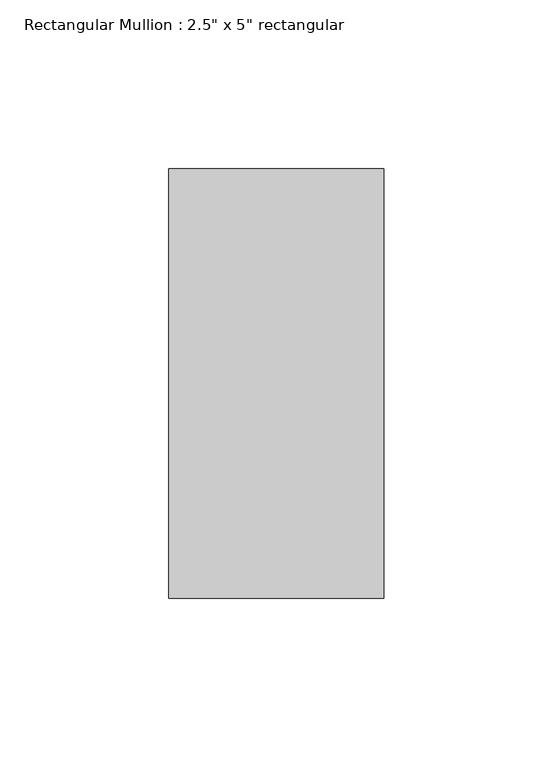
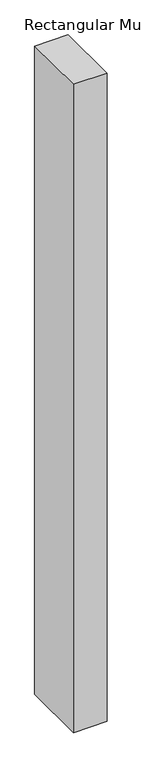
"""IFC4 building model written with IfcOpenShell, lengths in millimetres: member geometry."""

from ifc_helpers import new_model, si_unit, frame, origin, place, context, project, spatial, polyline, outline, extrude, source, transform, mapped, element, save


def member_9a0024e4(model_context):
    return source(origin(), model_context, "Body", "SweptSolid", [
        extrude(outline(polyline([(0.0, 63.5), (0.0, -63.5), (-63.5, -63.5), (-63.5, 63.5), (0.0, 63.5)])), frame((0.0, 0.0, -1299.6333333), z_axis=(0.0, 0.0, 1.0), x_axis=(1.0, 0.0, 0.0)), (0.0, 0.0, 1.0), 1299.6333333),
    ])


if __name__ == "__main__":
    model = new_model("IFC4")
    model_context = context("Model", 3, world=origin())
    ifc_project = project(units=[si_unit("LENGTHUNIT", "METRE", prefix="MILLI")], contexts=[model_context])
    site = spatial("IfcSite", under=ifc_project)
    building = spatial("IfcBuilding", under=site)
    placement = place(None, origin())
    member_shape = member_9a0024e4(model_context)
    element("IfcMember", 1, ObjectType="Rectangular Mullion : 2.5\" x 5\" rectangular", at=placement, inside=building, context=model_context, shape_type="MappedRepresentation", body=[
        mapped(member_shape, transform((0.0, 0.0, 0.0), x_axis=(1.0, 0.0, 0.0), y_axis=(0.0, 1.0, 0.0), z_axis=(0.0, 0.0, 1.0))),
    ])
    save(model, "model.ifc")

# Revit data of these elements
# Type "Rectangular Mullion : 2.5\" x 5\" rectangular"
#   built-in parameter 1007304 = 0.416667 (stored number, unit not read)
#   built-in parameter 1007301 = 0.104167 (stored number, unit not read)
#   built-in parameter 1007300 = 0.104167 (stored number, unit not read)
# Element 1 (IfcMember, "Rectangular Mullion : 2.5\" x 5\" rectangular")
#   Materials on its faces: "Aluminum"
# Materials
#   "Aluminum": class "Metal", colour RGB 247 247 247, transparency 0, Description = "Aluminum 6061", Cost = 0
